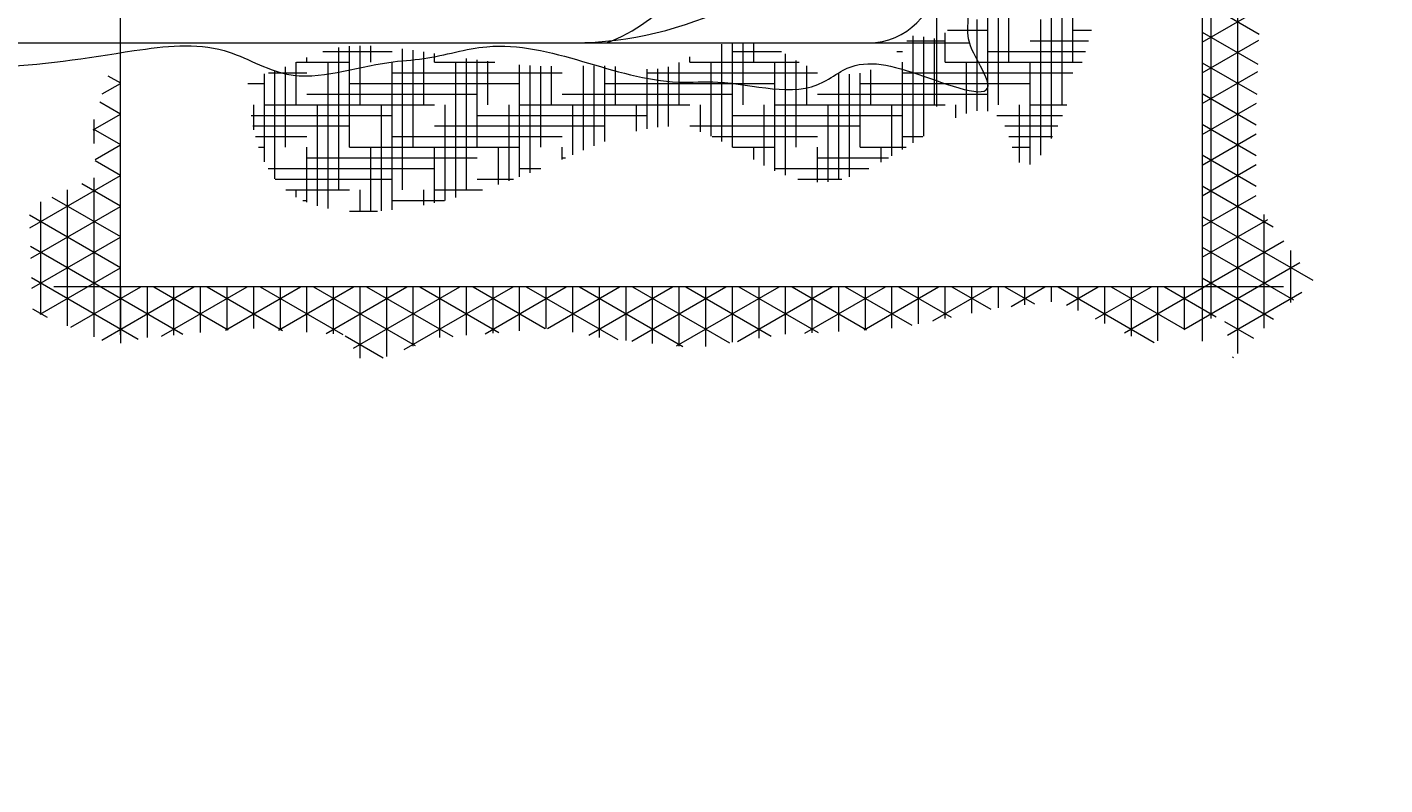
# Model space of a CAD drawing. Units: inches. Extents: x 2330 to 3943, y 1763 to 3461.
# Tile 16 of 40: x 3148 to 3231, y 2547 to 2593. Entities that reach past the tile are written whole.
import ezdxf

# ---------------------------------------------------------------- set-up
doc = ezdxf.new("R2010")
doc.units = ezdxf.units.IN
doc.layers.add('A-ANNO-DIMS', color=2, linetype='Continuous', lineweight=18)
doc.layers.add('A-FURN', color=8, linetype='Continuous', lineweight=13)
doc.styles.get("Standard").update_dxf_attribs({"font": 'arial.ttf'})
doc.dimstyles.get("Standard").update_dxf_attribs({"dimtxt": 0.18, "dimasz": 0.18, "dimexe": 0.18, "dimexo": 0.0625, "dimgap": 0.09, "dimtad": 0, "dimtih": 1, "dimtoh": 1, "dimdec": 4, "dimzin": 0, "dimdsep": 46, "dimtxsty": 'Standard', "dimcen": 0.09, "dimadec": 0, "dimazin": 0, "dimtfac": 1, "dimtdec": 4, "dimtofl": 0, "dimtmove": 0, "dimatfit": 3, "dimfxl": 1, "dimtolj": 1, "dimtzin": 0, "dimarcsym": 0})

# ---------------------------------------------------------------- blocks, each defined once
blk = doc.blocks.new('A$C200C7901')
for p, q in [((2.3121, 1.6596), (2.3121, 0.0201)), ((2, 0.2957), (2, 1.2957)), ((1.0407, 0.0275), (1.0407, 0.4323)), ((0.4061, 0.3703), (2.0386, 0.3703)), ((2.4073, 0.0839), (0.9625, 0.0839))]:
    blk.add_line(p, q)
at = {"linetype": 'ByBlock'}
for p, q in [((2.3224, 0.0468), (2.3224, 1.6627)), ((2.3224, 0.0468), (2.3224, 1.6627)), ((2.3537, 0.0056), (2.3537, 1.634)), ((2.3537, 0.0056), (2.3537, 1.634)), ((2.0849, 0.3477), (2.0849, 0.5477)), ((2.0849, 0.3477), (2.0849, 0.5477)), ((2.1599, 0.3477), (2.1599, 0.5477)), ((2.1599, 0.3477), (2.1599, 0.5477)), ((2.0724, 0.2977), (2.0724, 0.4977)), ((2.0724, 0.2977), (2.0724, 0.4977)), ((2.1474, 0.2977), (2.1474, 0.4977)), ((2.1474, 0.2977), (2.1474, 0.4977)), ((2.0599, 0.2903), (2.0599, 0.4477)), ((2.0599, 0.2903), (2.0599, 0.4477)), ((2.1349, 0.2582), (2.1349, 0.4477)), ((2.1349, 0.2582), (2.1349, 0.4477)), ((2.3121, 0.4191), (2.3789, 0.3805)), ((2.3121, 0.4191), (2.3789, 0.3805)), ((2.3121, 0.3711), (2.3801, 0.4103)), ((2.3121, 0.3711), (2.3801, 0.4103)), ((2.0127, 0.3852), (2.0599, 0.3852)), ((2.0127, 0.3852), (2.0599, 0.3852)), ((2.0474, 0.2905), (2.0474, 0.3977)), ((2.0474, 0.2905), (2.0474, 0.3977)), ((2.1224, 0.2385), (2.1224, 0.3977)), ((2.1224, 0.2385), (2.1224, 0.3977)), ((2.1599, 0.3852), (2.1819, 0.3852)), ((2.1599, 0.3852), (2.1819, 0.3852)), ((2.3121, 0.383), (2.3775, 0.3452)), ((2.3121, 0.383), (2.3775, 0.3452)), ((1.7474, 0.2546), (1.7474, 0.3689)), ((1.7474, 0.2546), (1.7474, 0.3689)), ((1.7599, 0.2477), (1.7599, 0.3703)), ((1.7599, 0.2477), (1.7599, 0.3703)), ((1.7724, 0.2977), (1.7724, 0.3703)), ((1.7724, 0.2977), (1.7724, 0.3703)), ((1.7849, 0.3477), (1.7849, 0.3703)), ((1.7849, 0.3477), (1.7849, 0.3703)), ((1.9648, 0.3727), (2.0099, 0.3727)), ((1.9648, 0.3727), (2.0099, 0.3727)), ((1.9724, 0.253), (1.9724, 0.3785)), ((1.9724, 0.253), (1.9724, 0.3785)), ((1.9849, 0.2609), (1.9849, 0.3774)), ((1.9849, 0.2609), (1.9849, 0.3774)), ((1.9974, 0.2977), (1.9974, 0.3753)), ((1.9974, 0.2977), (1.9974, 0.3753)), ((2.0099, 0.3477), (2.0099, 0.382)), ((2.0099, 0.3477), (2.0099, 0.382)), ((2.1099, 0.3727), (2.1784, 0.3727)), ((2.1099, 0.3727), (2.1784, 0.3727)), ((2.3121, 0.335), (2.3786, 0.3734)), ((2.3121, 0.335), (2.3786, 0.3734)), ((1.2599, 0.3477), (1.2599, 0.3531)), ((1.2599, 0.3477), (1.2599, 0.3531)), ((1.2785, 0.3602), (1.3599, 0.3602)), ((1.2785, 0.3602), (1.3599, 0.3602)), ((1.2974, 0.1977), (1.2974, 0.3647)), ((1.2974, 0.1977), (1.2974, 0.3647)), ((1.3099, 0.2477), (1.3099, 0.3663)), ((1.3099, 0.2477), (1.3099, 0.3663)), ((1.3224, 0.2977), (1.3224, 0.3669)), ((1.3224, 0.2977), (1.3224, 0.3669)), ((1.3349, 0.3477), (1.3349, 0.3668)), ((1.3349, 0.3477), (1.3349, 0.3668)), ((1.3724, 0.1977), (1.3724, 0.3634)), ((1.3724, 0.1977), (1.3724, 0.3634)), ((1.3849, 0.2477), (1.3849, 0.3616)), ((1.3849, 0.2477), (1.3849, 0.3616)), ((1.3974, 0.2977), (1.3974, 0.3597)), ((1.3974, 0.2977), (1.3974, 0.3597)), ((1.4099, 0.3477), (1.4099, 0.3578)), ((1.4099, 0.3477), (1.4099, 0.3578)), ((1.4474, 0.1977), (1.4474, 0.3521)), ((1.4474, 0.1977), (1.4474, 0.3521)), ((1.7099, 0.3477), (1.7099, 0.3539)), ((1.7099, 0.3477), (1.7099, 0.3539)), ((1.7599, 0.3602), (1.8177, 0.3602)), ((1.7599, 0.3602), (1.8177, 0.3602)), ((1.8224, 0.2148), (1.8224, 0.3575)), ((1.8224, 0.2148), (1.8224, 0.3575)), ((1.9532, 0.3602), (1.9599, 0.3602)), ((1.9532, 0.3602), (1.9599, 0.3602)), ((2.0599, 0.3602), (2.1747, 0.3602)), ((2.0599, 0.3602), (2.1747, 0.3602)), ((1.2148, 0.3352), (1.2599, 0.3352)), ((1.2148, 0.3352), (1.2599, 0.3352)), ((1.2224, 0.2106), (1.2224, 0.3375)), ((1.2224, 0.2106), (1.2224, 0.3375)), ((1.2349, 0.2477), (1.2349, 0.3422)), ((1.2349, 0.2477), (1.2349, 0.3422)), ((1.2474, 0.2977), (1.2474, 0.3476)), ((1.2474, 0.2977), (1.2474, 0.3476)), ((1.2475, 0.3477), (1.3099, 0.3477)), ((1.2475, 0.3477), (1.3099, 0.3477)), ((1.2849, 0.1758), (1.2849, 0.3477)), ((1.2849, 0.1758), (1.2849, 0.3477)), ((1.3599, 0.1741), (1.3599, 0.3477)), ((1.3599, 0.1741), (1.3599, 0.3477)), ((1.3599, 0.3352), (1.5599, 0.3352)), ((1.3599, 0.3352), (1.5599, 0.3352)), ((1.4099, 0.3477), (1.4806, 0.3477)), ((1.4099, 0.3477), (1.4806, 0.3477)), ((1.4349, 0.1886), (1.4349, 0.3477)), ((1.4349, 0.1886), (1.4349, 0.3477)), ((1.4599, 0.2477), (1.4599, 0.3504)), ((1.4599, 0.2477), (1.4599, 0.3504)), ((1.4724, 0.2977), (1.4724, 0.3487)), ((1.4724, 0.2977), (1.4724, 0.3487)), ((1.5099, 0.2129), (1.5099, 0.3447)), ((1.5099, 0.2129), (1.5099, 0.3447)), ((1.5224, 0.2177), (1.5224, 0.3438)), ((1.5224, 0.2177), (1.5224, 0.3438)), ((1.5349, 0.2477), (1.5349, 0.3431)), ((1.5349, 0.2477), (1.5349, 0.3431)), ((1.5474, 0.2977), (1.5474, 0.3428)), ((1.5474, 0.2977), (1.5474, 0.3428)), ((1.5849, 0.2443), (1.5849, 0.3434)), ((1.5849, 0.2443), (1.5849, 0.3434)), ((1.5974, 0.2496), (1.5974, 0.3435)), ((1.5974, 0.2496), (1.5974, 0.3435)), ((1.6099, 0.2546), (1.6099, 0.3432)), ((1.6099, 0.2546), (1.6099, 0.3432)), ((1.6224, 0.2977), (1.6224, 0.3424)), ((1.6224, 0.2977), (1.6224, 0.3424)), ((1.6599, 0.2695), (1.6599, 0.3394)), ((1.6599, 0.2695), (1.6599, 0.3394)), ((1.6599, 0.3352), (1.8599, 0.3352)), ((1.6599, 0.3352), (1.8599, 0.3352)), ((1.6724, 0.2713), (1.6724, 0.3398)), ((1.6724, 0.2713), (1.6724, 0.3398)), ((1.6849, 0.272), (1.6849, 0.3422)), ((1.6849, 0.272), (1.6849, 0.3422)), ((1.6974, 0.2977), (1.6974, 0.3472)), ((1.6974, 0.2977), (1.6974, 0.3472)), ((1.7099, 0.3477), (1.8383, 0.3477)), ((1.7099, 0.3477), (1.8383, 0.3477)), ((1.7349, 0.2607), (1.7349, 0.3477)), ((1.7349, 0.2607), (1.7349, 0.3477)), ((1.8099, 0.2201), (1.8099, 0.3477)), ((1.8099, 0.2201), (1.8099, 0.3477)), ((1.8349, 0.2477), (1.8349, 0.3497)), ((1.8349, 0.2477), (1.8349, 0.3497)), ((1.8474, 0.2977), (1.8474, 0.3432)), ((1.8474, 0.2977), (1.8474, 0.3432)), ((1.9224, 0.2977), (1.9224, 0.3385)), ((1.9224, 0.2977), (1.9224, 0.3385)), ((1.9599, 0.2452), (1.9599, 0.3477)), ((1.9599, 0.2452), (1.9599, 0.3477)), ((1.9599, 0.3352), (2.1599, 0.3352)), ((1.9599, 0.3352), (2.1599, 0.3352)), ((2.0099, 0.3477), (2.1708, 0.3477)), ((2.0099, 0.3477), (2.1708, 0.3477)), ((2.0349, 0.2874), (2.0349, 0.3477)), ((2.0349, 0.2874), (2.0349, 0.3477)), ((2.1099, 0.2274), (2.1099, 0.3477)), ((2.1099, 0.2274), (2.1099, 0.3477)), ((2.3121, 0.3469), (2.3761, 0.31)), ((2.3121, 0.3469), (2.3761, 0.31)), ((2.3121, 0.299), (2.3772, 0.3365)), ((2.3121, 0.299), (2.3772, 0.3365)), ((1.0194, 0.3103), (1.0407, 0.3227)), ((1.0194, 0.3103), (1.0407, 0.3227)), ((1.0261, 0.3316), (1.0407, 0.3232)), ((1.0261, 0.3316), (1.0407, 0.3232)), ((1.1904, 0.3227), (1.2099, 0.3227)), ((1.1904, 0.3227), (1.2099, 0.3227)), ((1.2099, 0.2308), (1.2099, 0.334)), ((1.2099, 0.2308), (1.2099, 0.334)), ((1.3099, 0.3227), (1.5099, 0.3227)), ((1.3099, 0.3227), (1.5099, 0.3227)), ((1.6099, 0.3227), (1.8099, 0.3227)), ((1.6099, 0.3227), (1.8099, 0.3227)), ((1.8849, 0.2093), (1.8849, 0.3337)), ((1.8849, 0.2093), (1.8849, 0.3337)), ((1.8974, 0.2129), (1.8974, 0.3335)), ((1.8974, 0.2129), (1.8974, 0.3335)), ((1.9099, 0.2477), (1.9099, 0.3349)), ((1.9099, 0.2477), (1.9099, 0.3349)), ((1.9099, 0.3227), (2.1099, 0.3227)), ((1.9099, 0.3227), (2.1099, 0.3227)), ((1.2599, 0.3102), (1.4599, 0.3102)), ((1.2599, 0.3102), (1.4599, 0.3102)), ((1.5599, 0.3102), (1.7599, 0.3102)), ((1.5599, 0.3102), (1.7599, 0.3102)), ((1.8599, 0.3102), (2.0599, 0.3102)), ((1.8599, 0.3102), (2.0599, 0.3102)), ((2.3121, 0.3108), (2.3755, 0.2742)), ((2.3121, 0.3108), (2.3755, 0.2742)), ((1.0164, 0.3011), (1.0407, 0.2871)), ((1.0164, 0.3011), (1.0407, 0.2871)), ((1.1974, 0.2683), (1.1974, 0.2977)), ((1.1974, 0.2683), (1.1974, 0.2977)), ((1.2099, 0.2977), (1.4099, 0.2977)), ((1.2099, 0.2977), (1.4099, 0.2977)), ((1.2724, 0.1788), (1.2724, 0.2977)), ((1.2724, 0.1788), (1.2724, 0.2977)), ((1.3474, 0.173), (1.3474, 0.2977)), ((1.3474, 0.173), (1.3474, 0.2977)), ((1.4224, 0.1854), (1.4224, 0.2977)), ((1.4224, 0.1854), (1.4224, 0.2977)), ((1.4974, 0.2083), (1.4974, 0.2977)), ((1.4974, 0.2083), (1.4974, 0.2977)), ((1.5099, 0.2977), (1.7099, 0.2977)), ((1.5099, 0.2977), (1.7099, 0.2977)), ((1.5724, 0.2389), (1.5724, 0.2977)), ((1.5724, 0.2389), (1.5724, 0.2977)), ((1.6474, 0.2668), (1.6474, 0.2977)), ((1.6474, 0.2668), (1.6474, 0.2977)), ((1.7224, 0.2658), (1.7224, 0.2977)), ((1.7224, 0.2658), (1.7224, 0.2977)), ((1.7974, 0.2263), (1.7974, 0.2977)), ((1.7974, 0.2263), (1.7974, 0.2977)), ((1.8099, 0.2977), (2.0099, 0.2977)), ((1.8099, 0.2977), (2.0099, 0.2977)), ((1.8724, 0.2072), (1.8724, 0.2977)), ((1.8724, 0.2072), (1.8724, 0.2977)), ((1.9474, 0.2376), (1.9474, 0.2977)), ((1.9474, 0.2376), (1.9474, 0.2977)), ((2.0224, 0.2822), (2.0224, 0.2977)), ((2.0224, 0.2822), (2.0224, 0.2977)), ((2.0974, 0.2299), (2.0974, 0.2977)), ((2.0974, 0.2299), (2.0974, 0.2977)), ((2.1099, 0.2977), (2.153, 0.2977)), ((2.1099, 0.2977), (2.153, 0.2977)), ((2.3121, 0.2629), (2.3757, 0.2996)), ((2.3121, 0.2629), (2.3757, 0.2996)), ((1.0089, 0.2682), (1.0407, 0.2866)), ((1.0089, 0.2682), (1.0407, 0.2866)), ((1.0099, 0.2521), (1.0099, 0.2804)), ((1.0099, 0.2521), (1.0099, 0.2804)), ((1.1943, 0.2852), (1.3599, 0.2852)), ((1.1943, 0.2852), (1.3599, 0.2852)), ((1.1965, 0.2727), (1.3099, 0.2727)), ((1.1965, 0.2727), (1.3099, 0.2727)), ((1.4099, 0.2727), (1.6099, 0.2727)), ((1.4099, 0.2727), (1.6099, 0.2727)), ((1.4599, 0.2852), (1.6599, 0.2852)), ((1.4599, 0.2852), (1.6599, 0.2852)), ((1.7099, 0.2727), (1.9099, 0.2727)), ((1.7099, 0.2727), (1.9099, 0.2727)), ((1.7599, 0.2852), (1.9599, 0.2852)), ((1.7599, 0.2852), (1.9599, 0.2852)), ((2.0708, 0.2852), (2.1478, 0.2852)), ((2.0708, 0.2852), (2.1478, 0.2852)), ((2.08, 0.2727), (2.1422, 0.2727)), ((2.08, 0.2727), (2.1422, 0.2727)), ((2.3121, 0.2747), (2.3755, 0.2381)), ((2.3121, 0.2747), (2.3755, 0.2381)), ((1.0088, 0.2694), (1.0407, 0.251)), ((1.0088, 0.2694), (1.0407, 0.251)), ((1.1994, 0.2602), (1.2599, 0.2602)), ((1.1994, 0.2602), (1.2599, 0.2602)), ((1.3599, 0.2602), (1.5599, 0.2602)), ((1.3599, 0.2602), (1.5599, 0.2602)), ((1.7361, 0.2602), (1.8599, 0.2602)), ((1.7361, 0.2602), (1.8599, 0.2602)), ((1.9599, 0.2602), (1.9838, 0.2602)), ((1.9599, 0.2602), (1.9838, 0.2602)), ((2.0848, 0.2602), (2.1359, 0.2602)), ((2.0848, 0.2602), (2.1359, 0.2602)), ((2.3121, 0.2268), (2.3755, 0.2634)), ((2.3121, 0.2268), (2.3755, 0.2634)), ((1.0111, 0.2334), (1.0407, 0.2505)), ((1.0111, 0.2334), (1.0407, 0.2505)), ((1.2031, 0.2477), (1.2099, 0.2477)), ((1.2031, 0.2477), (1.2099, 0.2477)), ((1.2599, 0.1831), (1.2599, 0.2477)), ((1.2599, 0.1831), (1.2599, 0.2477)), ((1.3099, 0.2477), (1.5099, 0.2477)), ((1.3099, 0.2477), (1.5099, 0.2477)), ((1.3349, 0.1723), (1.3349, 0.2477)), ((1.3349, 0.1723), (1.3349, 0.2477)), ((1.4099, 0.1825), (1.4099, 0.2477)), ((1.4099, 0.1825), (1.4099, 0.2477)), ((1.4849, 0.2039), (1.4849, 0.2477)), ((1.4849, 0.2039), (1.4849, 0.2477)), ((1.5599, 0.2335), (1.5599, 0.2477)), ((1.5599, 0.2335), (1.5599, 0.2477)), ((1.7599, 0.2477), (1.8099, 0.2477)), ((1.7599, 0.2477), (1.8099, 0.2477)), ((1.7849, 0.2332), (1.7849, 0.2477)), ((1.7849, 0.2332), (1.7849, 0.2477)), ((1.8599, 0.2068), (1.8599, 0.2477)), ((1.8599, 0.2068), (1.8599, 0.2477)), ((1.9099, 0.2477), (1.9639, 0.2477)), ((1.9099, 0.2477), (1.9639, 0.2477)), ((1.9349, 0.2304), (1.9349, 0.2477)), ((1.9349, 0.2304), (1.9349, 0.2477)), ((2.0888, 0.2477), (2.1099, 0.2477)), ((2.0888, 0.2477), (2.1099, 0.2477)), ((1.0112, 0.232), (1.0407, 0.215)), ((1.0112, 0.232), (1.0407, 0.215)), ((1.2599, 0.2352), (1.4599, 0.2352)), ((1.2599, 0.2352), (1.4599, 0.2352)), ((1.5599, 0.2352), (1.5638, 0.2352)), ((1.5599, 0.2352), (1.5638, 0.2352)), ((1.8599, 0.2352), (1.9433, 0.2352)), ((1.8599, 0.2352), (1.9433, 0.2352)), ((2.3121, 0.2387), (2.3755, 0.202)), ((2.3121, 0.2387), (2.3755, 0.202)), ((2.3121, 0.1907), (2.3755, 0.2273)), ((2.3121, 0.1907), (2.3755, 0.2273)), ((0.9344, 0.153), (1.0407, 0.2144)), ((0.9344, 0.153), (1.0407, 0.2144)), ((1.0099, 0.0251), (1.0099, 0.2117)), ((1.0099, 0.0251), (1.0099, 0.2117)), ((1.2142, 0.2227), (1.4099, 0.2227)), ((1.2142, 0.2227), (1.4099, 0.2227)), ((1.2227, 0.2102), (1.3599, 0.2102)), ((1.2227, 0.2102), (1.3599, 0.2102)), ((1.4599, 0.2102), (1.5027, 0.2102)), ((1.4599, 0.2102), (1.5027, 0.2102)), ((1.5099, 0.2227), (1.5346, 0.2227)), ((1.5099, 0.2227), (1.5346, 0.2227)), ((1.8099, 0.2227), (1.9203, 0.2227)), ((1.8099, 0.2227), (1.9203, 0.2227)), ((1.8368, 0.2102), (1.8884, 0.2102)), ((1.8368, 0.2102), (1.8884, 0.2102)), ((0.9787, 0.0381), (0.9787, 0.1976)), ((0.9787, 0.0381), (0.9787, 0.1976)), ((0.9953, 0.2051), (1.0407, 0.1789)), ((0.9953, 0.2051), (1.0407, 0.1789)), ((1.2351, 0.1977), (1.3099, 0.1977)), ((1.2351, 0.1977), (1.3099, 0.1977)), ((1.2474, 0.1892), (1.2474, 0.1977)), ((1.2474, 0.1892), (1.2474, 0.1977)), ((1.3224, 0.1722), (1.3224, 0.1977)), ((1.3224, 0.1722), (1.3224, 0.1977)), ((1.3974, 0.1799), (1.3974, 0.1977)), ((1.3974, 0.1799), (1.3974, 0.1977)), ((1.4099, 0.1977), (1.4662, 0.1977)), ((1.4099, 0.1977), (1.4662, 0.1977)), ((2.3121, 0.2026), (2.3953, 0.1545)), ((2.3121, 0.2026), (2.3953, 0.1545)), ((0.9355, 0.1176), (1.0407, 0.1783)), ((0.9355, 0.1176), (1.0407, 0.1783)), ((0.9474, 0.0512), (0.9474, 0.1835)), ((0.9474, 0.0512), (0.9474, 0.1835)), ((0.9602, 0.1893), (1.0407, 0.1428)), ((0.9602, 0.1893), (1.0407, 0.1428)), ((1.2552, 0.1852), (1.2599, 0.1852)), ((1.2552, 0.1852), (1.2599, 0.1852)), ((1.3599, 0.1852), (1.4215, 0.1852)), ((1.3599, 0.1852), (1.4215, 0.1852)), ((2.3121, 0.1546), (2.3755, 0.1912)), ((2.3121, 0.1546), (2.3755, 0.1912)), ((0.9339, 0.1684), (1.0407, 0.1067)), ((0.9339, 0.1684), (1.0407, 0.1067)), ((1.3099, 0.1727), (1.3428, 0.1727)), ((1.3099, 0.1727), (1.3428, 0.1727)), ((2.3121, 0.1665), (2.4419, 0.0916)), ((2.3121, 0.1665), (2.4419, 0.0916)), ((2.3121, 0.1185), (2.3891, 0.163)), ((2.3121, 0.1185), (2.3891, 0.163)), ((2.3849, 0.0355), (2.3849, 0.1686)), ((2.3849, 0.0355), (2.3849, 0.1686)), ((0.935, 0.1316), (1.114, 0.0283)), ((0.935, 0.1316), (1.114, 0.0283)), ((0.9366, 0.0822), (1.0407, 0.1422)), ((0.9366, 0.0822), (1.0407, 0.1422)), ((2.2208, 0.0297), (2.4078, 0.1377)), ((2.2208, 0.0297), (2.4078, 0.1377)), ((2.3121, 0.1304), (2.4193, 0.0685)), ((2.3121, 0.1304), (2.4193, 0.0685)), ((2.2903, 0.0337), (2.4265, 0.1124)), ((2.2903, 0.0337), (2.4265, 0.1124)), ((2.4162, 0.0655), (2.4162, 0.1264)), ((2.4162, 0.0655), (2.4162, 0.1264)), ((0.9463, 0.0516), (1.0407, 0.1061)), ((0.9463, 0.0516), (1.0407, 0.1061)), ((0.9362, 0.0948), (1.0616, 0.0225)), ((0.9362, 0.0948), (1.0616, 0.0225)), ((0.9826, 0.0365), (1.0647, 0.0839)), ((0.9826, 0.0365), (1.0647, 0.0839)), ((1.0189, 0.0214), (1.1272, 0.0839)), ((1.0189, 0.0214), (1.1272, 0.0839)), ((1.0412, 0.0179), (1.0412, 0.0839)), ((1.0412, 0.0179), (1.0412, 0.0839)), ((1.0724, 0.0243), (1.0724, 0.0839)), ((1.0724, 0.0243), (1.0724, 0.0839)), ((1.0801, 0.0839), (1.1675, 0.0335)), ((1.0801, 0.0839), (1.1675, 0.0335)), ((1.0891, 0.0259), (1.1897, 0.0839)), ((1.0891, 0.0259), (1.1897, 0.0839)), ((1.1037, 0.0273), (1.1037, 0.0839)), ((1.1037, 0.0273), (1.1037, 0.0839)), ((1.1349, 0.0303), (1.1349, 0.0839)), ((1.1349, 0.0303), (1.1349, 0.0839)), ((1.1426, 0.0839), (1.2313, 0.0327)), ((1.1426, 0.0839), (1.2313, 0.0327)), ((1.1642, 0.0331), (1.2522, 0.0839)), ((1.1642, 0.0331), (1.2522, 0.0839)), ((1.1662, 0.0333), (1.1662, 0.0839)), ((1.1662, 0.0333), (1.1662, 0.0839)), ((1.1974, 0.0351), (1.1974, 0.0839)), ((1.1974, 0.0351), (1.1974, 0.0839)), ((1.2051, 0.0839), (1.3023, 0.0278)), ((1.2051, 0.0839), (1.3023, 0.0278)), ((1.2266, 0.033), (1.3147, 0.0839)), ((1.2266, 0.033), (1.3147, 0.0839)), ((1.2287, 0.0329), (1.2287, 0.0839)), ((1.2287, 0.0329), (1.2287, 0.0839)), ((1.2599, 0.0308), (1.2599, 0.0839)), ((1.2599, 0.0308), (1.2599, 0.0839)), ((1.2676, 0.0839), (1.3871, 0.015)), ((1.2676, 0.0839), (1.3871, 0.015)), ((1.2824, 0.0292), (1.3772, 0.0839)), ((1.2824, 0.0292), (1.3772, 0.0839)), ((1.2912, 0.0286), (1.2912, 0.0839)), ((1.2912, 0.0286), (1.2912, 0.0839)), ((1.3146, 0.0117), (1.4397, 0.0839)), ((1.3146, 0.0117), (1.4397, 0.0839)), ((1.3224, 0), (1.3224, 0.0839)), ((1.3224, 0), (1.3224, 0.0839)), ((1.3301, 0.0839), (1.4312, 0.0256)), ((1.3301, 0.0839), (1.4312, 0.0256)), ((1.3537, 0.0022), (1.3537, 0.0839)), ((1.3537, 0.0022), (1.3537, 0.0839)), ((1.3743, 0.0101), (1.5022, 0.0839)), ((1.3743, 0.0101), (1.5022, 0.0839)), ((1.3849, 0.0141), (1.3849, 0.0839)), ((1.3849, 0.0141), (1.3849, 0.0839)), ((1.3926, 0.0839), (1.4856, 0.0302)), ((1.3926, 0.0839), (1.4856, 0.0302)), ((1.4162, 0.0243), (1.4162, 0.0839)), ((1.4162, 0.0243), (1.4162, 0.0839)), ((1.4474, 0.027), (1.4474, 0.0839)), ((1.4474, 0.027), (1.4474, 0.0839)), ((1.4551, 0.0839), (1.54, 0.0349)), ((1.4551, 0.0839), (1.54, 0.0349)), ((1.4693, 0.0288), (1.5647, 0.0839)), ((1.4693, 0.0288), (1.5647, 0.0839)), ((1.4787, 0.0296), (1.4787, 0.0839)), ((1.4787, 0.0296), (1.4787, 0.0839)), ((1.5099, 0.0323), (1.5099, 0.0839)), ((1.5099, 0.0323), (1.5099, 0.0839)), ((1.5176, 0.0839), (1.6251, 0.0219)), ((1.5176, 0.0839), (1.6251, 0.0219)), ((1.5412, 0.035), (1.5412, 0.0839)), ((1.5412, 0.035), (1.5412, 0.0839)), ((1.5427, 0.0351), (1.6272, 0.0839)), ((1.5427, 0.0351), (1.6272, 0.0839)), ((1.5724, 0.0308), (1.5724, 0.0839)), ((1.5724, 0.0308), (1.5724, 0.0839)), ((1.5801, 0.0839), (1.7018, 0.0137)), ((1.5801, 0.0839), (1.7018, 0.0137)), ((1.5911, 0.027), (1.6897, 0.0839)), ((1.5911, 0.027), (1.6897, 0.0839)), ((1.6037, 0.0245), (1.6037, 0.0839)), ((1.6037, 0.0245), (1.6037, 0.0839)), ((1.6349, 0.0208), (1.6349, 0.0839)), ((1.6349, 0.0208), (1.6349, 0.0839)), ((1.6416, 0.0201), (1.7522, 0.0839)), ((1.6416, 0.0201), (1.7522, 0.0839)), ((1.6426, 0.0839), (1.7565, 0.0182)), ((1.6426, 0.0839), (1.7565, 0.0182)), ((1.6662, 0.0175), (1.6662, 0.0839)), ((1.6662, 0.0175), (1.6662, 0.0839)), ((1.6944, 0.0145), (1.8147, 0.0839)), ((1.6944, 0.0145), (1.8147, 0.0839)), ((1.6974, 0.0141), (1.6974, 0.0839)), ((1.6974, 0.0141), (1.6974, 0.0839)), ((1.7051, 0.0839), (1.8054, 0.026)), ((1.7051, 0.0839), (1.8054, 0.026)), ((1.7287, 0.0137), (1.7287, 0.0839)), ((1.7287, 0.0137), (1.7287, 0.0839)), ((1.7599, 0.0187), (1.7599, 0.0839)), ((1.7599, 0.0187), (1.7599, 0.0839)), ((1.7659, 0.0197), (1.8772, 0.0839)), ((1.7659, 0.0197), (1.8772, 0.0839)), ((1.7676, 0.0839), (1.8606, 0.0303)), ((1.7676, 0.0839), (1.8606, 0.0303)), ((1.7912, 0.0237), (1.7912, 0.0839)), ((1.7912, 0.0237), (1.7912, 0.0839)), ((1.8224, 0.0281), (1.8224, 0.0839)), ((1.8224, 0.0281), (1.8224, 0.0839)), ((1.8301, 0.0839), (1.9175, 0.0335)), ((1.8301, 0.0839), (1.9175, 0.0335)), ((1.8452, 0.0294), (1.9397, 0.0839)), ((1.8452, 0.0294), (1.9397, 0.0839)), ((1.8537, 0.0299), (1.8537, 0.0839)), ((1.8537, 0.0299), (1.8537, 0.0839)), ((1.8849, 0.0316), (1.8849, 0.0839)), ((1.8849, 0.0316), (1.8849, 0.0839)), ((1.8926, 0.0839), (1.9706, 0.0389)), ((1.8926, 0.0839), (1.9706, 0.0389)), ((1.9146, 0.0333), (2.0022, 0.0839)), ((1.9146, 0.0333), (2.0022, 0.0839)), ((1.9162, 0.0334), (1.9162, 0.0839)), ((1.9162, 0.0334), (1.9162, 0.0839)), ((1.9474, 0.0352), (1.9474, 0.0839)), ((1.9474, 0.0352), (1.9474, 0.0839)), ((1.9551, 0.0839), (2.017, 0.0482)), ((1.9551, 0.0839), (2.017, 0.0482)), ((1.9787, 0.0405), (1.9787, 0.0839)), ((1.9787, 0.0405), (1.9787, 0.0839)), ((1.9953, 0.0438), (2.0647, 0.0839)), ((1.9953, 0.0438), (2.0647, 0.0839)), ((2.0099, 0.0468), (2.0099, 0.0839)), ((2.0099, 0.0468), (2.0099, 0.0839)), ((2.0176, 0.0839), (2.0634, 0.0575)), ((2.0176, 0.0839), (2.0634, 0.0575)), ((2.0412, 0.053), (2.0412, 0.0839)), ((2.0412, 0.053), (2.0412, 0.0839)), ((2.0724, 0.0592), (2.0724, 0.0839)), ((2.0724, 0.0592), (2.0724, 0.0839)), ((2.0801, 0.0839), (2.1147, 0.0639)), ((2.0801, 0.0839), (2.1147, 0.0639)), ((2.0873, 0.0609), (2.1272, 0.0839)), ((2.0873, 0.0609), (2.1272, 0.0839)), ((2.1037, 0.0627), (2.1037, 0.0839)), ((2.1037, 0.0627), (2.1037, 0.0839)), ((2.1349, 0.0662), (2.1349, 0.0839)), ((2.1349, 0.0662), (2.1349, 0.0839)), ((2.1426, 0.0839), (2.2557, 0.0186)), ((2.1426, 0.0839), (2.2557, 0.0186)), ((2.1526, 0.0625), (2.1897, 0.0839)), ((2.1526, 0.0625), (2.1897, 0.0839)), ((2.1662, 0.056), (2.1662, 0.0839)), ((2.1662, 0.056), (2.1662, 0.0839)), ((2.1867, 0.0461), (2.2522, 0.0839)), ((2.1867, 0.0461), (2.2522, 0.0839)), ((2.1974, 0.041), (2.1974, 0.0839)), ((2.1974, 0.041), (2.1974, 0.0839)), ((2.2051, 0.0839), (2.2913, 0.0342)), ((2.2051, 0.0839), (2.2913, 0.0342)), ((2.2287, 0.0259), (2.2287, 0.0839)), ((2.2287, 0.0259), (2.2287, 0.0839)), ((2.2599, 0.0205), (2.2599, 0.0839)), ((2.2599, 0.0205), (2.2599, 0.0839)), ((2.2676, 0.0839), (2.3285, 0.0488)), ((2.2676, 0.0839), (2.3285, 0.0488)), ((2.2912, 0.0341), (2.2912, 0.0839)), ((2.2912, 0.0341), (2.2912, 0.0839)), ((2.3121, 0.0943), (2.3958, 0.046)), ((2.3121, 0.0943), (2.3958, 0.046)), ((2.3417, 0.0273), (2.429, 0.0777)), ((2.3417, 0.0273), (2.429, 0.0777)), ((0.9374, 0.0581), (0.9545, 0.0482)), ((0.9374, 0.0581), (0.9545, 0.0482)), ((2.338, 0.0433), (2.3723, 0.0235)), ((2.338, 0.0433), (2.3723, 0.0235)), ((1.3048, 0.0264), (1.3494, 0.0006)), ((1.3048, 0.0264), (1.3494, 0.0006)), ((2.3476, 0.0017), (2.3488, 0.001)), ((2.3476, 0.0017), (2.3488, 0.001))]:
    blk.add_line(p, q, dxfattribs=at)
for centre, radius, start, end in [((1.5693, 0.8075), 0.4372, 269.0679, 9.9322), ((1.5372, 0.5659), 0.2094, 290.9415, 45.7647), ((1.92, 0.4503), 0.08, 270, 0)]:
    blk.add_arc(centre, radius, start, end)
blk.add_open_spline([(0.473, 1.2954), (0.4739, 1.2781), (0.4755, 1.2477), (0.5032, 1.2084), (0.4801, 1.1701), (0.4928, 1.1255), (0.4674, 1.0912), (0.4579, 1.0351), (0.501, 0.9724), (0.4311, 0.8832), (0.4902, 0.8637), (0.4843, 0.8288), (0.4774, 0.7906), (0.4625, 0.7457), (0.459, 0.6999), (0.4816, 0.6664), (0.4748, 0.625), (0.4791, 0.5889), (0.4533, 0.5528), (0.4738, 0.5004), (0.4658, 0.4502), (0.4696, 0.3946), (0.4189, 0.3935), (0.4493, 0.3684), (0.4694, 0.3857), (0.4922, 0.3576), (0.5297, 0.3262), (0.5917, 0.3353), (0.6454, 0.3754), (0.7083, 0.3741), (0.7643, 0.3328), (0.826, 0.346), (0.925, 0.3388), (1.0353, 0.3593), (1.1561, 0.3744), (1.2477, 0.3154), (1.3302, 0.3474), (1.4086, 0.3512), (1.5217, 0.3878), (1.6362, 0.3176), (1.7682, 0.3285), (1.8402, 0.3019), (1.9071, 0.3529), (1.9647, 0.3412), (2.0795, 0.2948), (2.0472, 0.3498), (2.0343, 0.3772), (2.0435, 0.43), (2.0109, 0.5782), (2.0746, 0.4643), (2.0805, 0.584), (2.0084, 0.5979), (2.0343, 0.6846), (2.0344, 0.746), (2.0293, 0.8096), (2.0489, 0.8545), (2.0652, 0.9218), (1.9842, 0.9297), (2.0007, 1.0162), (2.0367, 1.0585), (2.0367, 1.1102), (2.0457, 1.1647), (2.0226, 1.2084), (2.0234, 1.2306), (2.0236, 1.2352)], degree=3, knots=[0, 0, 0, 0, 51.660678, 90.967412, 128.902454, 170.303599, 219.852997, 247.834962, 336.321557, 429.35469, 458.821847, 477.222321, 524.135809, 581.038434, 617.839381, 657.146115, 693.947125, 740.178081, 760.753248, 820.731705, 885.133458, 928.777044, 953.563729, 976.574207, 995.553042, 1018.563482, 1064.584401, 1147.951297, 1174.787598, 1266.851571, 1308.018447, 1377.066427, 1441.511314, 1608.245014, 1714.11869, 1792.771707, 1913.247991, 1954.931389, 2029.864445, 2259.189419, 2305.221512, 2429.507982, 2456.344283, 2543.92595, 2627.925037, 2662.96218, 2687.736879, 2719.937755, 2839.540991, 2875.47895, 2953.681041, 2993.270313, 3066.872333, 3154.395764, 3200.397042, 3248.426375, 3312.828127, 3347.881398, 3444.484026, 3481.577522, 3518.665244, 3592.267265, 3644.719162, 3658.519501, 3658.519501, 3658.519501, 3658.519501], dxfattribs=at)
blk = doc.blocks.new('*D98')
at = {"layer": 'A-ANNO-DIMS', "color": 0, "lineweight": -2, "transparency": 16777216}
for p, q in [((3105.603, 2727.687), (3105.783, 2727.687)), ((3105.693, 2727.597), (3105.693, 2727.777)), ((3519.334, 2463.489), (3364.371, 2562.466)), ((3519.514, 2463.489), (3519.334, 2463.489))]:
    blk.add_line(p, q, dxfattribs=at)
at = {"layer": 'A-ANNO-DIMS', "color": 0, "transparency": 16777216}
blk.add_solid([(3364.387, 2562.491), (3364.355, 2562.441), (3364.219, 2562.563)], dxfattribs=at)
at = {"layer": 'Defpoints', "color": 0, "transparency": 16777216}
for p in [(3105.693, 2727.687), (3364.219, 2562.563)]:
    blk.add_point(p, dxfattribs=at)
at = {"layer": 'A-ANNO-DIMS', "color": 0, "transparency": 16777216, "insert": (3520.257, 2463.489), "char_height": 0.18, "attachment_point": 5}
blk.add_mtext('\\A1;3X R306.76', dxfattribs=at)

msp = doc.modelspace()

# ---------------------------------------------------------------- block references
at = {"layer": 'A-FURN', "xscale": 52.5181391560459, "yscale": 52.5181391560459, "zscale": 52.5181391560459}
msp.add_blockref('A$C200C7901', (3098.8053, 2572.8601), dxfattribs=at)

# ---------------------------------------------------------------- dimensions: what is measured, and where the dimension line sits
at = {"layer": 'A-ANNO-DIMS'}
dim = msp.add_radius_dim(center=(3105.6935, 2727.6869), mpoint=(3364.219, 2562.563), text='3X <>', dimstyle='Standard', override={"dimdec": 2, "dimlfac": 1, "dimrnd": 0, "dimzin": 0, "dimdsep": 46, "dimlunit": 2}, dxfattribs=at)
dim.commit()
dim.dimension.update_dxf_attribs({"geometry": '*D98', "text_midpoint": (3520.2574, 2463.4886), "dimtype": 164})

doc.saveas('drawing.dxf')
